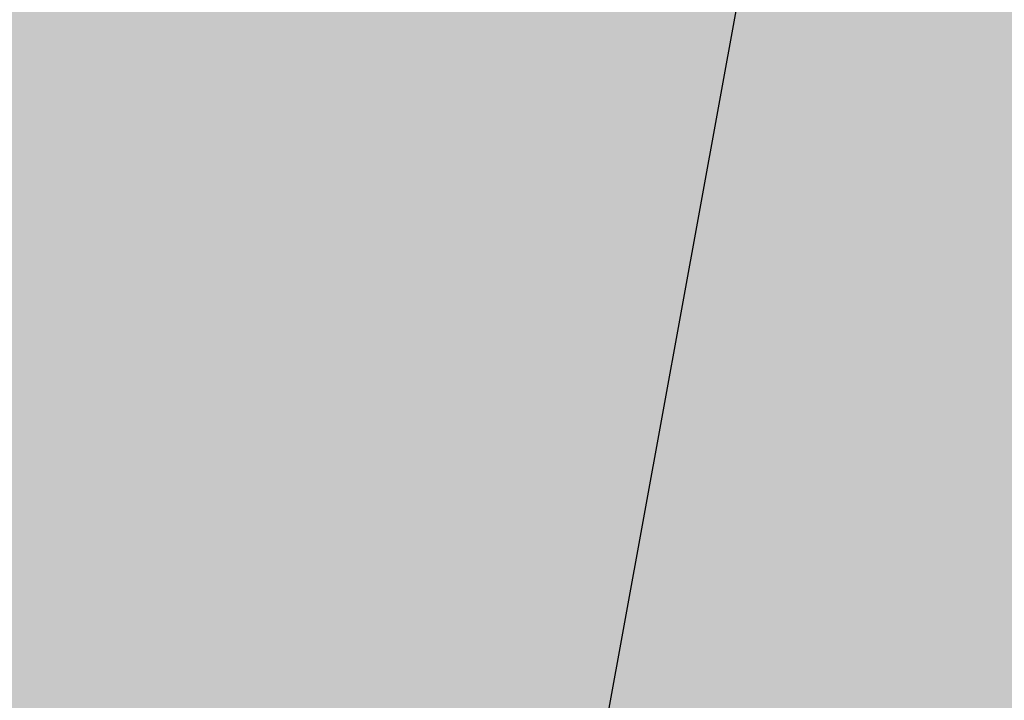
# Model space of a CAD drawing. Units: feet. Extents: x 3168 to 4724, y 827 to 1477.
# Tile 244 of 256: x 3383.8327 to 3384.7831, y 1098.344 to 1099.0007. Entities that reach past the tile are written whole.
import ezdxf

# ---------------------------------------------------------------- set-up
doc = ezdxf.new("R2010")
doc.units = ezdxf.units.FT
for name, color, linetype, lineweight in [('A-ELEV', 7, 'Continuous', 35), ('A-ELEV-PATT', 8, 'Continuous', 13), ('C-TOPO', 3, 'Continuous', 25)]:
    doc.layers.add(name, color=color, linetype=linetype, lineweight=lineweight)

msp = doc.modelspace()

# ---------------------------------------------------------------- hatches: boundary and pattern name
at = {"layer": 'A-ELEV-PATT'}
h = msp.add_hatch(color=256, dxfattribs=at)
h.dxf.hatch_style = 1
edge = h.paths.add_edge_path()
edge.add_ellipse((3552.90576, 979.22014), major_axis=(36.74492, 0), ratio=0.48484848, start_angle=0, end_angle=360)
edge = h.paths.add_edge_path()
edge.add_ellipse((3559.89164, 929.25228), major_axis=(36.74492, 0), ratio=0.48484848, start_angle=0, end_angle=360)
edge = h.paths.add_edge_path()
edge.add_line((3299.31681, 1198.60608), (3479.91671, 1198.60608))
edge.add_line((3479.91671, 1198.60608), (3479.91671, 1209.86857))
edge.add_spline(control_points=[(3479.91671, 1209.86857), (3464.30116, 1209.86857), (3448.6856, 1209.86857), (3410.94914, 1209.86857), (3388.82823, 1209.86857), (3355.64688, 1209.86857), (3344.58642, 1209.86857), (3327.99574, 1209.86857), (3322.46552, 1209.86857), (3314.17018, 1209.86857), (3311.40507, 1209.86857), (3307.2574, 1209.86857), (3305.87484, 1209.86857), (3303.801, 1209.86857), (3303.10973, 1209.86857), (3302.07281, 1209.86857), (3301.72717, 1209.86857), (3301.20871, 1209.86857), (3301.03589, 1209.86857), (3300.77666, 1209.86857), (3300.69025, 1209.86857), (3300.56064, 1209.86857), (3300.51743, 1209.86857), (3300.45263, 1209.86857), (3300.43102, 1209.86857), (3300.39862, 1209.86857), (3300.38782, 1209.86857), (3300.36622, 1209.86857), (3300.34568, 1209.86857), (3300.34555, 1209.86857), (3300.3455, 1209.86857), (3300.3433, 1209.86857), (3300.34115, 1209.86857), (3300.33791, 1209.86857), (3300.33683, 1209.86857), (3300.33394, 1209.86857), (3300.33213, 1209.86857), (3300.32552, 1209.86858), (3300.32071, 1209.86858), (3300.31092, 1209.86859), (3300.30595, 1209.8686), (3300.29051, 1209.86862), (3300.28005, 1209.86865), (3300.23243, 1209.86878), (3300.1953, 1209.86895), (3299.95107, 1209.87061), (3299.74482, 1209.87433), (3299.43683, 1209.88326), (3299.33439, 1209.88679), (3299.18108, 1209.89292), (3299.13003, 1209.8951), (3298.65222, 1209.9168), (3298.22946, 1209.94572), (3297.60163, 1210.00237), (3297.3934, 1210.02346), (3297.08265, 1210.05831), (3296.97933, 1210.07046), (3296.29295, 1210.15486), (3295.71815, 1210.24336), (3294.86872, 1210.39885), (3294.5877, 1210.45448), (3294.16934, 1210.54335), (3294.03042, 1210.57388), (3291.70715, 1211.1012), (3289.65359, 1211.81344), (3285.77626, 1213.56399), (3283.95141, 1214.60348), (3280.51216, 1216.98008), (3278.89724, 1218.31759), (3276.37991, 1220.82949), (3275.41604, 1221.91774), (3274.03934, 1223.7077), (3273.58104, 1224.34953), (3273.14323, 1225.01632)], knot_values=[39.119033, 39.119033, 39.119033, 39.119033, 39.286353, 39.286353, 39.523379, 39.523379, 39.641892, 39.641892, 39.701148, 39.701148, 39.730777, 39.730777, 39.745591, 39.745591, 39.752998, 39.752998, 39.756701, 39.756701, 39.758553, 39.758553, 39.759479, 39.759479, 39.759942, 39.759942, 39.760173, 39.760173, 39.760289, 39.760289, 39.760405, 39.760405, 39.760463, 39.760463, 39.763389, 39.763389, 39.764851, 39.764851, 39.767304, 39.767304, 39.773825, 39.773825, 39.78057, 39.78057, 39.79477, 39.79477, 39.845194, 39.845194, 40.126715, 40.126715, 40.267476, 40.267476, 40.337856, 40.337856, 40.927023, 40.927023, 41.221606, 41.221606, 41.368898, 41.368898, 42.202622, 42.202622, 42.619485, 42.619485, 42.827916, 42.827916, 46.118323, 46.118323, 49.408731, 49.408731, 52.699139, 52.699139, 54.927489, 54.927489, 56.104228, 56.104228, 56.104228, 56.104228], weights=[1, 1, 1, 1, 1, 1, 1, 1, 1, 1, 1, 1, 1, 1, 1, 1, 1, 1, 1, 1, 1, 1, 1, 1, 1, 1, 1, 1, 1, 1, 1, 1, 1, 1, 1, 1, 1, 1, 1, 1, 1, 1, 1, 1, 1, 1, 1, 1, 1, 1, 1, 1, 1, 1, 1, 1, 1, 1, 1, 1, 1, 1, 1, 1, 1, 1, 1, 1, 1, 1, 1, 1, 1, 1], degree=3, periodic=0)
edge.add_line((3273.14323, 1225.01632), (3273.14323, 1099.01632))
edge.add_line((3273.14323, 1099.01632), (3299.31681, 1099.01632))
edge.add_line((3299.31681, 1099.01632), (3299.31681, 1198.60608))
edge = h.paths.add_edge_path()
edge.add_line((3304.75844, 1324.15806), (3479.91671, 1324.15806))
edge.add_line((3479.91671, 1324.15806), (3479.91671, 1335.71462))
edge.add_line((3479.91671, 1335.71462), (3269.16163, 1335.71462))
edge.add_spline(control_points=[(3269.16163, 1335.71462), (3264.02423, 1335.71462), (3258.36412, 1328.95819), (3259.26431, 1323.90027)], knot_values=[0, 0, 0, 0, 15.412191, 15.412191, 15.412191, 15.412191], degree=3, periodic=0)
edge.add_line((3259.26431, 1323.90027), (3265.51685, 1288.76913))
edge.add_line((3265.51685, 1288.76913), (3275.2651, 1261.54563))
edge.add_line((3275.2651, 1261.54563), (3304.75844, 1261.54563))
edge.add_line((3304.75844, 1261.54563), (3304.75844, 1324.15806))
h = msp.add_hatch(color=256, dxfattribs=at)
h.dxf.hatch_style = 1
h.paths.add_polyline_path([(3384.52525, 1099.01632), (3335.02917, 1099.01632), (3299.31681, 1099.01632), (3273.14323, 1099.01632), (3217.56536, 1099.01632), (3168.06928, 827.11626), (3335.02917, 827.11626)])
h = msp.add_hatch(color=256, dxfattribs=at)
h.dxf.hatch_style = 1
h.paths.add_polyline_path([(3845.37573, 1099.01632), (3706.28837, 1099.01632), (3715.61866, 1081.39554), (3715.61866, 1052.31017), (3792.05516, 907.95566), (3463.22209, 903.64246), (3462.89922, 928.25741, 0.540152), (3462.89922, 1014.08264), (3621.89866, 1014.08264), (3601.65698, 1052.31017), (3601.65698, 1081.39554), (3592.32668, 1099.01632), (3384.52525, 1099.01632), (3335.02917, 827.11626), (3845.37573, 827.11626)])

# ---------------------------------------------------------------- linework, layer by layer
at = {"layer": 'A-ELEV'}
msp.add_open_spline([(3808.5202, 1099.01632), (3808.5202, 1141.41324), (3808.5202, 1183.81015), (3808.5202, 1226.63532), (3808.5202, 1227.06358), (3808.5202, 1227.49183), (3811.49187, 1248.99467), (3814.46354, 1270.49752), (3817.46523, 1292.21756), (3817.49525, 1292.43476), (3817.52526, 1292.65196), (3817.5728, 1310.10675), (3817.62034, 1327.56153), (3817.66788, 1345.01632), (3817.66788, 1345.45796), (3817.66788, 1345.89961), (3817.66788, 1346.45605), (3817.66788, 1346.57084), (3817.66788, 1346.75289), (3817.66788, 1346.82014), (3817.66788, 1346.93487), (3817.66788, 1346.98234), (3817.66788, 1347.03859), (3817.66788, 1347.04736), (3817.66788, 1347.07366), (3817.66788, 1347.0593), (3817.66788, 1347.06155), (3817.66788, 1347.06267), (3817.66788, 1347.06603), (3817.66787, 1347.06827), (3817.66787, 1347.075), (3817.66787, 1347.07949), (3817.66785, 1347.09294), (3817.66783, 1347.1019), (3817.66777, 1347.12879), (3817.6677, 1347.1467), (3817.66743, 1347.20042), (3817.66716, 1347.23619), (3817.6661, 1347.34338), (3817.66504, 1347.41469), (3817.66081, 1347.62809), (3817.65661, 1347.76971), (3817.63997, 1348.19249), (3817.62351, 1348.47159), (3817.55909, 1349.30007), (3817.49612, 1349.84059), (3817.25543, 1351.42416), (3817.02632, 1352.42879), (3816.30687, 1354.88891), (3815.74375, 1356.26873), (3814.46396, 1358.81921), (3813.74641, 1359.99097), (3812.19584, 1362.17234), (3811.36225, 1363.18212), (3809.58884, 1365.06901), (3808.64882, 1365.94611), (3806.65426, 1367.57962), (3805.5997, 1368.33615), (3803.35289, 1369.72233), (3802.16054, 1370.35239), (3799.60081, 1371.45359), (3798.23269, 1371.92548), (3795.28008, 1372.63462), (3793.69315, 1372.87207), (3791.86944, 1372.92648), (3791.74086, 1372.92922), (3791.35337, 1372.9341), (3791.09271, 1372.9329), (3790.30412, 1372.91507), (3789.76954, 1372.88419), (3789.20919, 1372.83024), (3789.19062, 1372.82842), (3789.13489, 1372.82291), (3789.0977, 1372.81914), (3789.04844, 1372.81401), (3789.0364, 1372.81274), (3789.00026, 1372.80892), (3788.97615, 1372.80633), (3788.9494, 1372.8034), (3788.94679, 1372.80312), (3788.94257, 1372.80266), (3788.94097, 1372.80248), (3788.93857, 1372.80222), (3788.93778, 1372.80213), (3788.93539, 1372.80187), (3788.86753, 1372.7944), (3788.75687, 1372.78223), (3788.70153, 1372.77614), (3788.53553, 1372.75788), (3788.42486, 1372.74571), (3788.09286, 1372.70918), (3787.87152, 1372.68484), (3787.20751, 1372.61179), (3786.76483, 1372.5631), (3785.43681, 1372.41701), (3784.55147, 1372.31962), (3781.89542, 1372.02744), (3780.12473, 1371.83266), (3774.81265, 1371.24831), (3771.27126, 1370.85874), (3760.64709, 1369.69004), (3753.56431, 1368.9109), (3732.31597, 1366.5735), (3718.15042, 1365.01523), (3694.00676, 1362.35933), (3684.02866, 1361.26169), (3674.05056, 1360.16406), (3664.60066, 1360.16406), (3655.15077, 1360.16406), (3626.80108, 1360.16406), (3607.90129, 1360.16406), (3551.20192, 1360.16406), (3513.40234, 1360.16406), (3467.72518, 1360.16406), (3459.8476, 1360.16406), (3436.21487, 1360.16406), (3420.45972, 1360.16406), (3373.19425, 1360.16406), (3341.68395, 1360.16406), (3302.84816, 1360.16406), (3295.52269, 1360.16406), (3286.03829, 1360.16406), (3283.87937, 1360.16406), (3277.40261, 1360.16406), (3273.08477, 1360.16406), (3267.73285, 1360.16406), (3266.69877, 1360.16406), (3263.59652, 1360.16406), (3261.52835, 1360.16406), (3259.23694, 1360.16406), (3259.0137, 1360.16406), (3258.34396, 1360.16406), (3257.89747, 1360.16406), (3257.431, 1360.16406), (3257.41102, 1360.16406), (3257.37057, 1360.16406), (3257.37547, 1360.16406), (3257.3746, 1360.16406), (3257.37394, 1360.16406), (3257.37196, 1360.16406), (3257.37064, 1360.16406), (3257.36667, 1360.16406), (3257.36403, 1360.16406), (3257.35611, 1360.16405), (3257.35083, 1360.16405), (3257.33499, 1360.16402), (3257.32443, 1360.164), (3257.29277, 1360.1639), (3257.27168, 1360.1638), (3257.20844, 1360.1634), (3257.16634, 1360.163), (3257.04021, 1360.16139), (3256.95635, 1360.15978), (3256.7055, 1360.15339), (3256.53924, 1360.14704), (3256.04357, 1360.12192), (3255.7173, 1360.0971), (3254.75245, 1360.00048), (3254.12797, 1359.90651), (3252.18007, 1359.52533), (3250.94157, 1359.14399), (3248.67018, 1358.24329), (3247.63574, 1357.72383), (3245.73263, 1356.60347), (3244.86339, 1356.00206), (3243.25311, 1354.74287), (3242.51197, 1354.08473), (3240.75105, 1352.34478), (3239.80096, 1351.22957), (3238.08777, 1348.87244), (3237.32469, 1347.63036), (3235.98251, 1344.97163), (3235.40221, 1343.55491), (3234.59108, 1340.81546), (3234.31088, 1339.54355), (3233.97649, 1336.80256), (3233.92211, 1335.33088), (3234.14892, 1332.59127), (3234.34953, 1331.3672), (3234.71989, 1329.99937), (3234.75242, 1329.88336), (3234.85362, 1329.5348), (3234.92589, 1329.30168), (3235.02484, 1329.00255), (3235.04692, 1328.93693), (3235.07764, 1328.84724), (3235.08592, 1328.8232), (3235.11094, 1328.75106), (3235.12783, 1328.70296), (3235.14799, 1328.64624), (3235.15106, 1328.63763), (3235.1561, 1328.62353), (3235.15806, 1328.61803), (3235.16021, 1328.61203), (3235.16561, 1328.59694), (3235.1801, 1328.55649), (3235.19026, 1328.5281), (3235.22076, 1328.44295), (3235.24108, 1328.38618), (3235.30207, 1328.21587), (3235.34273, 1328.10232), (3235.4647, 1327.7617), (3235.54601, 1327.53462), (3235.78995, 1326.85338), (3235.95258, 1326.39922), (3236.44046, 1325.03674), (3236.76571, 1324.12841), (3237.74148, 1321.40345), (3238.39198, 1319.5868), (3240.34351, 1314.13687), (3241.64452, 1310.50358), (3245.54757, 1299.60371), (3248.14961, 1292.33713), (3255.95571, 1270.53739), (3261.15977, 1256.00423), (3267.38762, 1238.612), (3268.4114, 1235.75294), (3269.51038, 1232.68386), (3269.58558, 1232.47385), (3269.70661, 1232.13585), (3269.75244, 1232.00786), (3269.82733, 1231.79873), (3269.85638, 1231.7176), (3269.90632, 1231.57812), (3269.92721, 1231.51978), (3269.97247, 1231.39341), (3269.99683, 1231.32537), (3270.0265, 1231.24251), (3270.03181, 1231.22768), (3270.04028, 1231.20402), (3270.03922, 1231.20698), (3270.03936, 1231.2066), (3270.03943, 1231.20641), (3270.03963, 1231.20585), (3270.03977, 1231.20547), (3270.04017, 1231.20433), (3270.04044, 1231.20358), (3270.04125, 1231.20131), (3270.0418, 1231.1998), (3270.04342, 1231.19527), (3270.0445, 1231.19225), (3270.04776, 1231.18318), (3270.04993, 1231.17714), (3270.05644, 1231.15903), (3270.06079, 1231.14696), (3270.07387, 1231.11076), (3270.08261, 1231.08666), (3270.10894, 1231.01441), (3270.1266, 1230.96635), (3270.17993, 1230.82246), (3270.21595, 1230.72692), (3270.32532, 1230.44151), (3270.40003, 1230.25281), (3270.62925, 1229.69144), (3270.78888, 1229.3235), (3271.28649, 1228.23832), (3271.6431, 1227.53975), (3272.77586, 1225.51528), (3273.61417, 1224.2605), (3275.41604, 1221.91774), (3276.37991, 1220.82949), (3278.89724, 1218.31759), (3280.51216, 1216.98008), (3283.95141, 1214.60348), (3285.77626, 1213.56399), (3289.65359, 1211.81344), (3291.70715, 1211.1012), (3294.03042, 1210.57388), (3294.16934, 1210.54335), (3294.5877, 1210.45448), (3294.86872, 1210.39885), (3295.71815, 1210.24336), (3296.29295, 1210.15486), (3296.97933, 1210.07046), (3297.08265, 1210.05831), (3297.3934, 1210.02346), (3297.60163, 1210.00237), (3298.22946, 1209.94572), (3298.65222, 1209.9168), (3299.13003, 1209.8951), (3299.18108, 1209.89292), (3299.33439, 1209.88679), (3299.43683, 1209.88326), (3299.74482, 1209.87433), (3299.95107, 1209.87061), (3300.1953, 1209.86895), (3300.23243, 1209.86878), (3300.28005, 1209.86865), (3300.29051, 1209.86862), (3300.30595, 1209.8686), (3300.31092, 1209.86859), (3300.32071, 1209.86858), (3300.32552, 1209.86858), (3300.33213, 1209.86857), (3300.33394, 1209.86857), (3300.33683, 1209.86857), (3300.33791, 1209.86857), (3300.34115, 1209.86857), (3300.3433, 1209.86857), (3300.3455, 1209.86857), (3300.34555, 1209.86857), (3300.34568, 1209.86857), (3300.36622, 1209.86857), (3300.38782, 1209.86857), (3300.39862, 1209.86857), (3300.43102, 1209.86857), (3300.45263, 1209.86857), (3300.51743, 1209.86857), (3300.56064, 1209.86857), (3300.69025, 1209.86857), (3300.77666, 1209.86857), (3301.03589, 1209.86857), (3301.20871, 1209.86857), (3301.72717, 1209.86857), (3302.07281, 1209.86857), (3303.10973, 1209.86857), (3303.801, 1209.86857), (3305.87484, 1209.86857), (3307.2574, 1209.86857), (3311.40507, 1209.86857), (3314.17018, 1209.86857), (3322.46552, 1209.86857), (3327.99574, 1209.86857), (3344.58642, 1209.86857), (3355.64688, 1209.86857), (3388.82823, 1209.86857), (3410.94914, 1209.86857), (3477.31185, 1209.86857), (3521.55366, 1209.86857), (3566.83618, 1209.86857), (3567.87689, 1209.86857), (3570.99902, 1209.86857), (3573.08043, 1209.86857), (3575.7814, 1209.86857), (3576.40094, 1209.86857), (3577.29582, 1209.86857), (3577.57115, 1209.86857), (3578.39715, 1209.86857), (3578.94781, 1209.86857), (3579.75649, 1209.86857), (3580.01451, 1209.86857), (3580.34274, 1209.86857), (3580.32686, 1209.86857), (3580.32717, 1209.86857), (3580.32732, 1209.86857), (3580.32778, 1209.86857), (3580.32809, 1209.86857), (3580.329, 1209.86857), (3580.32961, 1209.86857), (3580.33145, 1209.86857), (3580.33267, 1209.86857), (3580.33633, 1209.86857), (3580.33878, 1209.86857), (3580.34611, 1209.86856), (3580.35099, 1209.86856), (3580.36566, 1209.86854), (3580.37544, 1209.86852), (3580.4048, 1209.86845), (3580.42439, 1209.86838), (3580.48318, 1209.86808), (3580.52244, 1209.86779), (3580.64036, 1209.86662), (3580.71919, 1209.86545), (3580.95632, 1209.86077), (3581.11522, 1209.85607), (3581.59416, 1209.83723), (3581.91642, 1209.81833), (3582.88995, 1209.74243), (3583.54799, 1209.66617), (3585.53183, 1209.36062), (3586.86722, 1209.05389), (3589.47155, 1208.25247), (3590.74024, 1207.75785), (3591.99545, 1207.1588), (3592.05781, 1207.12874), (3592.24424, 1207.03795), (3592.36768, 1206.97663), (3592.73528, 1206.79036), (3592.97675, 1206.6631), (3593.24454, 1206.51644), (3593.27473, 1206.49982), (3593.36512, 1206.44984), (3593.42511, 1206.41633), (3593.60431, 1206.31529), (3593.72273, 1206.24721), (3593.85721, 1206.1684), (3593.87436, 1206.15832), (3593.92574, 1206.12804), (3593.9599, 1206.1078), (3594.06209, 1206.0469), (3594.12983, 1206.00607), (3594.20844, 1205.95817), (3594.21968, 1205.9513), (3594.25339, 1205.93069), (3594.27582, 1205.91692), (3594.34297, 1205.87554), (3594.38756, 1205.84785), (3594.43362, 1205.81905), (3594.43526, 1205.81802), (3594.44017, 1205.81495), (3594.44345, 1205.81289), (3594.44712, 1205.81059), (3594.44752, 1205.81035), (3594.44869, 1205.80961), (3594.44948, 1205.80912), (3594.45037, 1205.80856), (3594.45047, 1205.8085), (3594.4506, 1205.80842), (3594.4674, 1205.79789), (3594.49327, 1205.78167), (3594.5062, 1205.77357), (3594.54501, 1205.74925), (3594.57088, 1205.73303), (3594.64849, 1205.6844), (3594.70023, 1205.65197), (3594.85544, 1205.55469), (3594.95892, 1205.48984), (3595.26936, 1205.29528), (3595.47631, 1205.16558), (3596.09719, 1204.77646), (3596.5111, 1204.51705), (3597.75284, 1203.73883), (3598.58067, 1203.22001), (3601.06415, 1201.66355), (3602.71981, 1200.62591), (3607.68677, 1197.513), (3610.99809, 1195.43773), (3620.93202, 1189.2119), (3627.55464, 1185.06135), (3647.42251, 1172.60971), (3660.66775, 1164.30861), (3700.40348, 1139.40531), (3726.89397, 1122.80312), (3757.20572, 1103.80605), (3761.02697, 1101.41118), (3764.84822, 1099.01632), (3745.32827, 1099.01632), (3725.80832, 1099.01632), (3706.28837, 1099.01632), (3706.28837, 1108.45324), (3706.28837, 1117.89016), (3706.28837, 1127.32708), (3710.75075, 1127.32708), (3715.21314, 1127.32708), (3719.67553, 1127.32708)], degree=3, knots=[0, 0, 0, 0, 0.982037, 0.982037, 0.991957, 0.991957, 0.991957, 1.966522, 1.966522, 1.976367, 1.976367, 1.976367, 2.976367, 2.976367, 2.976367, 3.00169, 3.00169, 3.008272, 3.008272, 3.012129, 3.012129, 3.014851, 3.014851, 3.015353, 3.015353, 3.016359, 3.016359, 3.017365, 3.017365, 3.019376, 3.019376, 3.023398, 3.023398, 3.031442, 3.031442, 3.047531, 3.047531, 3.079708, 3.079708, 3.144063, 3.144063, 3.272772, 3.272772, 3.53019, 3.53019, 4.045026, 4.045026, 5.074698, 5.074698, 6.700878, 6.700878, 8.327058, 8.327058, 9.953238, 9.953238, 11.579418, 11.579418, 13.205598, 13.205598, 14.831778, 14.831778, 16.457958, 16.457958, 18.084138, 18.084138, 18.206872, 18.206872, 18.45234, 18.45234, 18.943275, 18.943275, 18.960093, 18.960093, 18.993729, 18.993729, 19.00461, 19.00461, 19.026374, 19.026374, 19.028737, 19.028737, 19.03018, 19.03018, 19.030897, 19.030897, 19.032332, 19.032332, 19.033766, 19.033766, 19.036636, 19.036636, 19.042374, 19.042374, 19.053851, 19.053851, 19.076805, 19.076805, 19.122714, 19.122714, 19.21453, 19.21453, 19.398163, 19.398163, 19.765429, 19.765429, 20.024128, 20.024128, 20.024128, 20.092031, 20.092031, 20.227836, 20.227836, 20.499446, 20.499446, 20.556051, 20.556051, 20.66926, 20.66926, 20.895678, 20.895678, 20.948316, 20.948316, 20.963829, 20.963829, 20.994855, 20.994855, 21.002285, 21.002285, 21.017146, 21.017146, 21.01875, 21.01875, 21.021959, 21.021959, 21.022102, 21.022102, 21.022249, 21.022249, 21.022708, 21.022708, 21.023627, 21.023627, 21.025464, 21.025464, 21.029138, 21.029138, 21.036486, 21.036486, 21.051183, 21.051183, 21.080575, 21.080575, 21.139361, 21.139361, 21.256932, 21.256932, 21.492073, 21.492073, 21.962356, 21.962356, 23.01002, 23.01002, 24.057684, 24.057684, 25.105348, 25.105348, 26.153011, 26.153011, 27.776787, 27.776787, 29.400562, 29.400562, 31.024337, 31.024337, 32.278801, 32.278801, 33.533265, 33.533265, 34.467568, 34.467568, 34.553971, 34.553971, 34.726776, 34.726776, 34.775309, 34.775309, 34.793079, 34.793079, 34.82862, 34.82862, 34.834979, 34.834979, 34.839039, 34.839039, 34.839411, 34.839411, 34.840285, 34.840285, 34.842034, 34.842034, 34.845531, 34.845531, 34.852525, 34.852525, 34.866512, 34.866512, 34.894488, 34.894488, 34.950439, 34.950439, 35.062342, 35.062342, 35.286147, 35.286147, 35.733758, 35.733758, 35.821815, 35.821815, 35.828283, 35.828283, 35.832225, 35.832225, 35.834724, 35.834724, 35.836521, 35.836521, 35.838617, 35.838617, 35.839073, 35.839073, 35.839345, 35.839345, 35.839617, 35.839617, 35.840161, 35.840161, 35.841249, 35.841249, 35.843425, 35.843425, 35.847778, 35.847778, 35.856482, 35.856482, 35.873891, 35.873891, 35.908709, 35.908709, 35.978345, 35.978345, 36.117617, 36.117617, 36.396161, 36.396161, 36.953248, 36.953248, 38.067423, 38.067423, 40.295772, 40.295772, 42.524122, 42.524122, 45.81453, 45.81453, 49.104937, 49.104937, 52.395345, 52.395345, 52.603776, 52.603776, 53.020639, 53.020639, 53.854363, 53.854363, 54.001655, 54.001655, 54.296238, 54.296238, 54.885405, 54.885405, 54.955785, 54.955785, 55.096546, 55.096546, 55.378067, 55.378067, 55.42849, 55.42849, 55.442691, 55.442691, 55.449436, 55.449436, 55.455957, 55.455957, 55.458409, 55.458409, 55.459872, 55.459872, 55.462798, 55.462798, 55.462856, 55.462856, 55.462972, 55.462972, 55.463088, 55.463088, 55.463319, 55.463319, 55.463782, 55.463782, 55.464708, 55.464708, 55.46656, 55.46656, 55.470263, 55.470263, 55.47767, 55.47767, 55.492484, 55.492484, 55.522112, 55.522112, 55.581369, 55.581369, 55.699882, 55.699882, 55.936907, 55.936907, 56.410959, 56.410959, 56.42211, 56.42211, 56.444413, 56.444413, 56.451051, 56.451051, 56.454001, 56.454001, 56.459901, 56.459901, 56.462666, 56.462666, 56.463418, 56.463418, 56.464171, 56.464171, 56.465675, 56.465675, 56.468684, 56.468684, 56.474702, 56.474702, 56.486738, 56.486738, 56.51081, 56.51081, 56.558955, 56.558955, 56.655243, 56.655243, 56.847821, 56.847821, 57.232975, 57.232975, 58.003284, 58.003284, 59.543901, 59.543901, 62.625137, 62.625137, 68.787607, 68.787607, 74.950078, 74.950078, 75.27336, 75.27336, 75.919923, 75.919923, 77.213051, 77.213051, 77.377769, 77.377769, 77.707206, 77.707206, 78.366079, 78.366079, 78.462532, 78.462532, 78.655436, 78.655436, 79.041245, 79.041245, 79.105735, 79.105735, 79.234714, 79.234714, 79.492672, 79.492672, 79.502197, 79.502197, 79.521249, 79.521249, 79.523534, 79.523534, 79.528103, 79.528103, 79.528682, 79.528682, 79.528885, 79.528885, 79.529089, 79.529089, 79.529495, 79.529495, 79.530308, 79.530308, 79.531935, 79.531935, 79.535187, 79.535187, 79.541693, 79.541693, 79.554704, 79.554704, 79.580725, 79.580725, 79.632769, 79.632769, 79.736856, 79.736856, 79.94503, 79.94503, 80.361377, 80.361377, 80.421435, 80.421435, 80.421435, 81.421435, 81.421435, 81.421435, 82.421435, 82.421435, 82.421435, 83.421435, 83.421435, 83.421435, 83.421435], dxfattribs=at)
at = {"layer": 'C-TOPO'}
msp.add_line((3384.52525, 1099.01632), (3335.02917, 827.11626), dxfattribs=at)
msp.add_lwpolyline([(3384.52525, 1099.01632), (3335.02917, 827.11626), (3845.37573, 827.11626), (3845.37573, 1099.01632), (3335.02917, 1099.01632)], dxfattribs=at)

doc.saveas('drawing.dxf')
